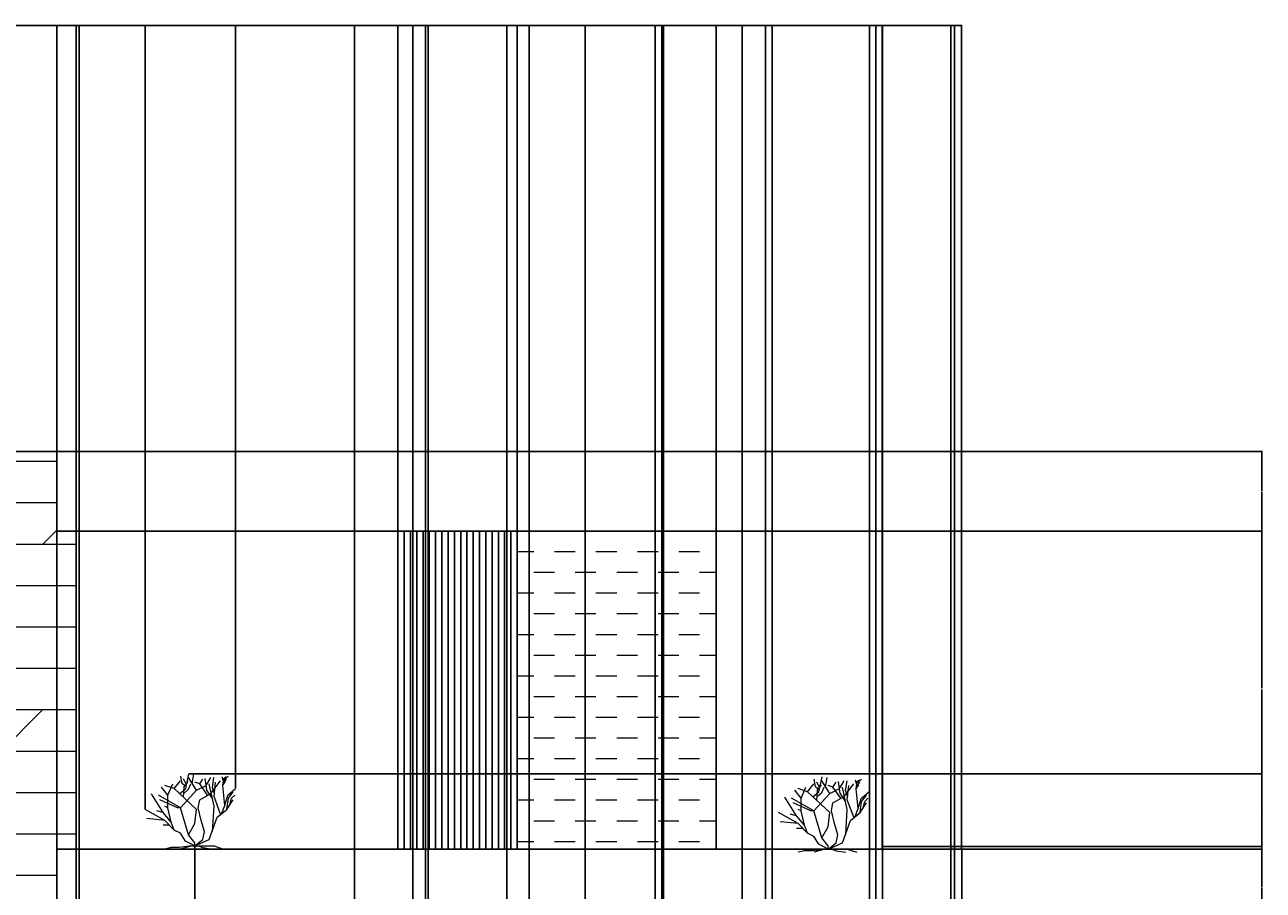
# Model space of a CAD drawing. Units: inches. Extents: x 250 to 1217, y -42 to 832.
# Tile 7 of 7: x 670 to 1043, y 571 to 832. Entities that reach past the tile are written whole.
import ezdxf

# ---------------------------------------------------------------- set-up
doc = ezdxf.new("R2010")
doc.units = ezdxf.units.IN
doc.header["$MEASUREMENT"] = 0
for name, color, linetype, lineweight in [('A-ANNO-DIMS', 2, 'Continuous', 18), ('A-ELEV', 7, 'Continuous', 25), ('A-ELEV-PATT', 8, 'Continuous', 13), ('L-PLNT', 3, 'Continuous', 13)]:
    doc.layers.add(name, color=color, linetype=linetype, lineweight=lineweight)
doc.styles.get("Standard").update_dxf_attribs({"font": 'arial.ttf'})
doc.dimstyles.get("Standard").update_dxf_attribs({"dimtxt": 0.18, "dimasz": 0.18, "dimexe": 0.18, "dimexo": 0.0625, "dimgap": 0.09, "dimtad": 0, "dimtih": 1, "dimtoh": 1, "dimdec": 4, "dimzin": 0, "dimdsep": 46, "dimtxsty": 'Standard', "dimcen": 0.09, "dimadec": 0, "dimazin": 0, "dimtfac": 1, "dimtdec": 4, "dimtofl": 0, "dimtmove": 0, "dimatfit": 3, "dimfxl": 1, "dimtolj": 1, "dimtzin": 0, "dimarcsym": 0})

# ---------------------------------------------------------------- blocks, each defined once
blk = doc.blocks.new('*U2')
for p, q in [((-11.433, 18.289), (-10.457, 22.749)), ((-9.48, 19.775), (-8.992, 22.592)), ((-16.8, 16.32), (-18.72, 18.72)), ((-14.88, 18.24), (-17.76, 19.2)), ((-16.8, 16.32), (-15.36, 19.68)), ((-14.88, 18.24), (-12.96, 20.64)), ((-12.471, 19.775), (-12.898, 22.044)), ((-11.677, 19.071), (-12.471, 19.775)), ((-11.28, 19.619), (-12.104, 21.184)), ((-12.043, 15.628), (-11.921, 18.836)), ((-11.921, 18.836), (-10.64, 20.401)), ((-10.579, 18.054), (-9.846, 19.697)), ((-8.16, 17.76), (-10.56, 21.6)), ((-7.2, 19.68), (-8.64, 20.16)), ((-8.16, 17.76), (-5.28, 19.2)), ((-7.2, 19.68), (-6.24, 21.12)), ((-4.8, 16.32), (-7.2, 19.68)), ((-5.086, 17.741), (-5.513, 21.34)), ((-5.28, 19.2), (-3.84, 21.6)), ((-2.88, 12.96), (-4.32, 19.68)), ((-3.84, 16.8), (-0.96, 20.64)), ((-3.377, 18.602), (-2.888, 21.575)), ((-2.88, 15.84), (-2.4, 20.16)), ((-0.508, 21.888), (-0.081, 20.558)), ((-0.203, 19.149), (0.102, 21.34)), ((0.346, 13.203), (-0.203, 19.149)), ((-0.142, 19.384), (0.59, 20.401)), ((-0.02, 20.01), (0.896, 21.105)), ((0.041, 20.714), (1.384, 22.044)), ((0.102, 21.34), (0.835, 21.888)), ((-18.24, 11.04), (-21.755, 16.655)), ((-12.96, 12.48), (-19.68, 16.32)), ((-16.8, 12.48), (-16.8, 16.32)), ((-8.16, 12), (-14.88, 18.24)), ((-13.325, 16.724), (-11.433, 18.289)), ((-12.96, 12.48), (-8.16, 17.76)), ((-11.982, 16.802), (-10.579, 18.054)), ((-7.2, 14.88), (-3.84, 16.8)), ((-3.377, 15.315), (-5.086, 17.819)), ((-2.766, 16.802), (-3.377, 18.602)), ((-0.96, 10.56), (-2.88, 15.84)), ((0.346, 13.203), (1.323, 16.254)), ((0.96, 12), (1.44, 15.36)), ((1.323, 16.254), (3.642, 18.289)), ((1.44, 15.36), (2.88, 17.28)), ((1.92, 13.44), (2.4, 15.36)), ((2.4, 15.36), (3.36, 16.32)), ((-17.76, 8.64), (-23.663, 11.961)), ((-18.24, 11.04), (-20.16, 11.52)), ((-13.92, 12.48), (-19.2, 14.88)), ((-16.8, 12.48), (-17.76, 12.96)), ((-15.84, 8.16), (-16.8, 12.48)), ((-12.96, 12.48), (-13.92, 12.48)), ((-10.56, 4.32), (-12.96, 12.48)), ((-8.64, 7.68), (-8.16, 12)), ((-7.68, 12.48), (-7.2, 14.88)), ((-6.72, 8.64), (-7.68, 12.48)), ((-3.36, 5.28), (-2.88, 12.96)), ((-1.92, 9.6), (0.96, 12)), ((-0.48, 10.8), (0.346, 13.203)), ((0.96, 12), (2.88, 14.88)), ((-17.76, 8.64), (-23.128, 9.222)), ((-15.84, 8.16), (-18.24, 11.04)), ((-14.88, 5.76), (-17.76, 8.64)), ((-14.88, 5.76), (-15.84, 8.16)), ((-10.56, 4.32), (-8.64, 7.68)), ((-5.76, 5.28), (-6.72, 8.64)), ((-4.32, 2.88), (-1.92, 9.6)), ((-16.32, 7.2), (-18.24, 7.2)), ((-12.96, 4.8), (-14.88, 5.76)), ((-11.52, 2.4), (-12.96, 4.8)), ((-8.64, 1.92), (-10.56, 4.32)), ((-6.24, 2.88), (-5.76, 5.28)), ((-15.84, 0.48), (-17.76, 0)), ((-13.44, 0.48), (-15.84, 0.48)), ((-9.6, 0.96), (-13.44, 0.48)), ((-9.6, 0.96), (-12.96, 0)), ((-8.64, 0.96), (-11.52, 2.4)), ((-9.6, 0.96), (-7.68, 0.96)), ((-8.64, 0.96), (-4.32, 2.88)), ((-8.64, 0.96), (-6.24, 2.88)), ((-8.64, 0.96), (-8.64, 1.92)), ((-8.64, 0.96), (-2.88, 0.96)), ((-7.68, 0.96), (-6.24, 0.48)), ((-6.24, 0.48), (-3.36, 0)), ((-2.88, 0.96), (0, 0))]:
    blk.add_line(p, q)
blk = doc.blocks.new('*D9')
at = {"layer": 'A-ANNO-DIMS', "color": 0, "lineweight": -2, "transparency": 16777216}
for p, q in [((630.78, 702.99), (630.78, 831.77)), ((630.96, 831.59), (654.6, 831.59)), ((679.01, 831.59), (655.36, 831.59)), ((679.19, 702.99), (679.19, 831.77))]:
    blk.add_line(p, q, dxfattribs=at)
at = {"layer": 'A-ANNO-DIMS', "color": 0, "transparency": 16777216}
for points in [[(630.96, 831.62), (630.96, 831.56), (630.78, 831.59)], [(679.01, 831.62), (679.01, 831.56), (679.19, 831.59)]]:
    blk.add_solid(points, dxfattribs=at)
at = {"layer": 'Defpoints', "color": 0, "transparency": 16777216}
for p in [(679.19, 831.59), (630.78, 702.93), (679.19, 702.93)]:
    blk.add_point(p, dxfattribs=at)
at = {"layer": 'A-ANNO-DIMS', "color": 0, "transparency": 16777216, "insert": (654.98, 831.59), "char_height": 0.18, "attachment_point": 5}
blk.add_mtext('\\A1;48.41', dxfattribs=at)
blk = doc.blocks.new('*D10')
at = {"layer": 'A-ANNO-DIMS', "color": 0, "lineweight": -2, "transparency": 16777216}
for p, q in [((679.19, 702.99), (679.19, 831.77)), ((679.37, 831.59), (815.24, 831.59)), ((952.05, 831.59), (816.18, 831.59)), ((952.23, 702.99), (952.23, 831.77))]:
    blk.add_line(p, q, dxfattribs=at)
at = {"layer": 'A-ANNO-DIMS', "color": 0, "transparency": 16777216}
for points in [[(679.37, 831.62), (679.37, 831.56), (679.19, 831.59)], [(952.05, 831.62), (952.05, 831.56), (952.23, 831.59)]]:
    blk.add_solid(points, dxfattribs=at)
at = {"layer": 'Defpoints', "color": 0, "transparency": 16777216}
for p in [(952.23, 831.59), (679.19, 702.93), (952.23, 702.93)]:
    blk.add_point(p, dxfattribs=at)
at = {"layer": 'A-ANNO-DIMS', "color": 0, "transparency": 16777216, "insert": (815.71, 831.59), "char_height": 0.18, "attachment_point": 5}
blk.add_mtext('\\A1;273.05', dxfattribs=at)
blk = doc.blocks.new('*D19')
at = {"layer": 'A-ANNO-DIMS', "color": 0, "lineweight": -2, "transparency": 16777216}
for p, q in [((928.21, 583.67), (1043.08, 583.67)), ((1042.9, 583.49), (1042.9, 571.48)), ((1042.9, 559.11), (1042.9, 571.12)), ((952.41, 558.93), (1043.08, 558.93))]:
    blk.add_line(p, q, dxfattribs=at)
at = {"layer": 'A-ANNO-DIMS', "color": 0, "transparency": 16777216}
for points in [[(1042.87, 583.49), (1042.93, 583.49), (1042.9, 583.67)], [(1042.87, 559.11), (1042.93, 559.11), (1042.9, 558.93)]]:
    blk.add_solid(points, dxfattribs=at)
at = {"layer": 'Defpoints', "color": 0, "transparency": 16777216}
for p in [(928.15, 583.67), (1042.9, 583.67), (952.34, 558.93)]:
    blk.add_point(p, dxfattribs=at)
at = {"layer": 'A-ANNO-DIMS', "color": 0, "transparency": 16777216, "insert": (1042.9, 571.3), "char_height": 0.18, "attachment_point": 5}
blk.add_mtext('\\A1;24.747', dxfattribs=at)
blk = doc.blocks.new('*D20')
at = {"layer": 'A-ANNO-DIMS', "color": 0, "lineweight": -2, "transparency": 16777216}
for p, q in [((928.3, 678.93), (1043.08, 678.93)), ((1042.9, 678.75), (1042.9, 631.48)), ((1042.9, 583.85), (1042.9, 631.12)), ((928.21, 583.67), (1043.08, 583.67))]:
    blk.add_line(p, q, dxfattribs=at)
at = {"layer": 'A-ANNO-DIMS', "color": 0, "transparency": 16777216}
for points in [[(1042.87, 678.75), (1042.93, 678.75), (1042.9, 678.93)], [(1042.87, 583.85), (1042.93, 583.85), (1042.9, 583.67)]]:
    blk.add_solid(points, dxfattribs=at)
at = {"layer": 'Defpoints', "color": 0, "transparency": 16777216}
for p in [(928.23, 678.93), (1042.9, 678.93), (928.15, 583.67)]:
    blk.add_point(p, dxfattribs=at)
at = {"layer": 'A-ANNO-DIMS', "color": 0, "transparency": 16777216, "insert": (1042.9, 631.3), "char_height": 0.18, "attachment_point": 5}
blk.add_mtext('\\A1;95.25', dxfattribs=at)
blk = doc.blocks.new('*D21')
at = {"layer": 'A-ANNO-DIMS', "color": 0, "lineweight": -2, "transparency": 16777216}
for p, q in [((952.3, 702.93), (1043.08, 702.93)), ((1042.9, 702.75), (1042.9, 691.11)), ((1042.9, 679.11), (1042.9, 690.75)), ((928.3, 678.93), (1043.08, 678.93))]:
    blk.add_line(p, q, dxfattribs=at)
at = {"layer": 'A-ANNO-DIMS', "color": 0, "transparency": 16777216}
for points in [[(1042.87, 702.75), (1042.93, 702.75), (1042.9, 702.93)], [(1042.87, 679.11), (1042.93, 679.11), (1042.9, 678.93)]]:
    blk.add_solid(points, dxfattribs=at)
at = {"layer": 'Defpoints', "color": 0, "transparency": 16777216}
for p in [(952.23, 702.93), (1042.9, 702.93), (928.23, 678.93)]:
    blk.add_point(p, dxfattribs=at)
at = {"layer": 'A-ANNO-DIMS', "color": 0, "transparency": 16777216, "insert": (1042.9, 690.93), "char_height": 0.18, "attachment_point": 5}
blk.add_mtext('\\A1;24', dxfattribs=at)
blk = doc.blocks.new('*D27')
at = {"layer": 'A-ANNO-DIMS', "color": 0, "lineweight": -2, "transparency": 16777216}
for p, q in [((624.98, 174.99), (624.98, 831.77)), ((625.16, 831.59), (655.07, 831.59)), ((685.76, 831.59), (655.86, 831.59)), ((685.94, 176.49), (685.94, 831.77))]:
    blk.add_line(p, q, dxfattribs=at)
at = {"layer": 'A-ANNO-DIMS', "color": 0, "transparency": 16777216}
for points in [[(625.16, 831.62), (625.16, 831.56), (624.98, 831.59)], [(685.76, 831.62), (685.76, 831.56), (685.94, 831.59)]]:
    blk.add_solid(points, dxfattribs=at)
at = {"layer": 'Defpoints', "color": 0, "transparency": 16777216}
for p in [(685.94, 831.59), (685.94, 176.43), (624.98, 174.93)]:
    blk.add_point(p, dxfattribs=at)
at = {"layer": 'A-ANNO-DIMS', "color": 0, "transparency": 16777216, "insert": (655.46, 831.59), "char_height": 0.18, "attachment_point": 5}
blk.add_mtext('\\A1;60.96', dxfattribs=at)
blk = doc.blocks.new('*D28')
at = {"layer": 'A-ANNO-DIMS', "color": 0, "lineweight": -2, "transparency": 16777216}
for p, q in [((685.94, 176.49), (685.94, 831.77)), ((686.12, 831.59), (727.07, 831.59)), ((768.8, 831.59), (727.86, 831.59)), ((768.98, 162.99), (768.98, 831.77))]:
    blk.add_line(p, q, dxfattribs=at)
at = {"layer": 'A-ANNO-DIMS', "color": 0, "transparency": 16777216}
for points in [[(686.12, 831.62), (686.12, 831.56), (685.94, 831.59)], [(768.8, 831.62), (768.8, 831.56), (768.98, 831.59)]]:
    blk.add_solid(points, dxfattribs=at)
at = {"layer": 'Defpoints', "color": 0, "transparency": 16777216}
for p in [(768.98, 831.59), (685.94, 176.43), (768.98, 162.93)]:
    blk.add_point(p, dxfattribs=at)
at = {"layer": 'A-ANNO-DIMS', "color": 0, "transparency": 16777216, "insert": (727.46, 831.59), "char_height": 0.18, "attachment_point": 5}
blk.add_mtext('\\A1;83.04', dxfattribs=at)
blk = doc.blocks.new('*D29')
at = {"layer": 'A-ANNO-DIMS', "color": 0, "lineweight": -2, "transparency": 16777216}
for p, q in [((768.98, 162.99), (768.98, 831.77)), ((769.16, 831.59), (779.67, 831.59)), ((791.11, 831.59), (780.6, 831.59)), ((791.29, 174.99), (791.29, 831.77))]:
    blk.add_line(p, q, dxfattribs=at)
at = {"layer": 'A-ANNO-DIMS', "color": 0, "transparency": 16777216}
for points in [[(769.16, 831.62), (769.16, 831.56), (768.98, 831.59)], [(791.11, 831.62), (791.11, 831.56), (791.29, 831.59)]]:
    blk.add_solid(points, dxfattribs=at)
at = {"layer": 'Defpoints', "color": 0, "transparency": 16777216}
for p in [(791.29, 831.59), (791.29, 174.93), (768.98, 162.93)]:
    blk.add_point(p, dxfattribs=at)
at = {"layer": 'A-ANNO-DIMS', "color": 0, "transparency": 16777216, "insert": (780.13, 831.59), "char_height": 0.18, "attachment_point": 5}
blk.add_mtext('\\A1;22.303', dxfattribs=at)
blk = doc.blocks.new('*D30')
at = {"layer": 'A-ANNO-DIMS', "color": 0, "lineweight": -2, "transparency": 16777216}
for p, q in [((814.96, 174.99), (814.96, 831.77)), ((815.14, 831.59), (826.33, 831.59)), ((838.45, 831.59), (827.26, 831.59)), ((838.63, 174.99), (838.63, 831.77))]:
    blk.add_line(p, q, dxfattribs=at)
at = {"layer": 'A-ANNO-DIMS', "color": 0, "transparency": 16777216}
for points in [[(815.14, 831.62), (815.14, 831.56), (814.96, 831.59)], [(838.45, 831.62), (838.45, 831.56), (838.63, 831.59)]]:
    blk.add_solid(points, dxfattribs=at)
at = {"layer": 'Defpoints', "color": 0, "transparency": 16777216}
for p in [(838.63, 831.59), (814.96, 174.93), (838.63, 174.93)]:
    blk.add_point(p, dxfattribs=at)
at = {"layer": 'A-ANNO-DIMS', "color": 0, "transparency": 16777216, "insert": (826.8, 831.59), "char_height": 0.18, "attachment_point": 5}
blk.add_mtext('\\A1;23.674', dxfattribs=at)
blk = doc.blocks.new('*D31')
at = {"layer": 'A-ANNO-DIMS', "color": 0, "lineweight": -2, "transparency": 16777216}
for p, q in [((862.31, 174.99), (862.31, 831.77)), ((862.49, 831.59), (873.68, 831.59)), ((885.8, 831.59), (874.61, 831.59)), ((885.98, 174.99), (885.98, 831.77))]:
    blk.add_line(p, q, dxfattribs=at)
at = {"layer": 'A-ANNO-DIMS', "color": 0, "transparency": 16777216}
for points in [[(862.49, 831.62), (862.49, 831.56), (862.31, 831.59)], [(885.8, 831.62), (885.8, 831.56), (885.98, 831.59)]]:
    blk.add_solid(points, dxfattribs=at)
at = {"layer": 'Defpoints', "color": 0, "transparency": 16777216}
for p in [(885.98, 831.59), (862.31, 174.93), (885.98, 174.93)]:
    blk.add_point(p, dxfattribs=at)
at = {"layer": 'A-ANNO-DIMS', "color": 0, "transparency": 16777216, "insert": (874.15, 831.59), "char_height": 0.18, "attachment_point": 5}
blk.add_mtext('\\A1;23.674', dxfattribs=at)
blk = doc.blocks.new('*D32')
at = {"layer": 'A-ANNO-DIMS', "color": 0, "lineweight": -2, "transparency": 16777216}
for p, q in [((885.98, 174.99), (885.98, 831.77)), ((886.16, 831.59), (917.26, 831.59)), ((948.8, 831.59), (917.7, 831.59)), ((948.98, 174.99), (948.98, 831.77))]:
    blk.add_line(p, q, dxfattribs=at)
at = {"layer": 'A-ANNO-DIMS', "color": 0, "transparency": 16777216}
for points in [[(886.16, 831.62), (886.16, 831.56), (885.98, 831.59)], [(948.8, 831.62), (948.8, 831.56), (948.98, 831.59)]]:
    blk.add_solid(points, dxfattribs=at)
at = {"layer": 'Defpoints', "color": 0, "transparency": 16777216}
for p in [(948.98, 831.59), (885.98, 174.93), (948.98, 174.93)]:
    blk.add_point(p, dxfattribs=at)
at = {"layer": 'A-ANNO-DIMS', "color": 0, "transparency": 16777216, "insert": (917.48, 831.59), "char_height": 0.18, "attachment_point": 5}
blk.add_mtext('\\A1;63', dxfattribs=at)
blk = doc.blocks.new('*D33')
at = {"layer": 'A-ANNO-DIMS', "color": 0, "lineweight": -2, "transparency": 16777216}
for p, q in [((791.29, 414.99), (791.29, 831.77)), ((791.47, 831.59), (802.66, 831.59)), ((814.78, 831.59), (803.59, 831.59)), ((814.96, 414.99), (814.96, 831.77))]:
    blk.add_line(p, q, dxfattribs=at)
at = {"layer": 'A-ANNO-DIMS', "color": 0, "transparency": 16777216}
for points in [[(791.47, 831.62), (791.47, 831.56), (791.29, 831.59)], [(814.78, 831.62), (814.78, 831.56), (814.96, 831.59)]]:
    blk.add_solid(points, dxfattribs=at)
at = {"layer": 'Defpoints', "color": 0, "transparency": 16777216}
for p in [(814.96, 831.59), (791.29, 414.93), (814.96, 414.93)]:
    blk.add_point(p, dxfattribs=at)
at = {"layer": 'A-ANNO-DIMS', "color": 0, "transparency": 16777216, "insert": (803.12, 831.59), "char_height": 0.18, "attachment_point": 5}
blk.add_mtext('\\A1;23.674', dxfattribs=at)
blk = doc.blocks.new('*D34')
at = {"layer": 'A-ANNO-DIMS', "color": 0, "lineweight": -2, "transparency": 16777216}
for p, q in [((838.63, 414.99), (838.63, 831.77)), ((838.81, 831.59), (850.01, 831.59)), ((862.13, 831.59), (850.94, 831.59)), ((862.31, 414.99), (862.31, 831.77))]:
    blk.add_line(p, q, dxfattribs=at)
at = {"layer": 'A-ANNO-DIMS', "color": 0, "transparency": 16777216}
for points in [[(838.81, 831.62), (838.81, 831.56), (838.63, 831.59)], [(862.13, 831.62), (862.13, 831.56), (862.31, 831.59)]]:
    blk.add_solid(points, dxfattribs=at)
at = {"layer": 'Defpoints', "color": 0, "transparency": 16777216}
for p in [(862.31, 831.59), (838.63, 414.93), (862.31, 414.93)]:
    blk.add_point(p, dxfattribs=at)
at = {"layer": 'A-ANNO-DIMS', "color": 0, "transparency": 16777216, "insert": (850.47, 831.59), "char_height": 0.18, "attachment_point": 5}
blk.add_mtext('\\A1;23.674', dxfattribs=at)
blk = doc.blocks.new('*D45')
at = {"layer": 'A-ANNO-DIMS', "color": 0, "lineweight": -2, "transparency": 16777216}
for p, q in [((685.06, 678.99), (685.06, 831.77)), ((685.24, 831.59), (733.21, 831.59)), ((781.95, 831.59), (733.99, 831.59)), ((782.13, 678.99), (782.13, 831.77))]:
    blk.add_line(p, q, dxfattribs=at)
at = {"layer": 'A-ANNO-DIMS', "color": 0, "transparency": 16777216}
for points in [[(685.24, 831.62), (685.24, 831.56), (685.06, 831.59)], [(781.95, 831.62), (781.95, 831.56), (782.13, 831.59)]]:
    blk.add_solid(points, dxfattribs=at)
at = {"layer": 'Defpoints', "color": 0, "transparency": 16777216}
for p in [(782.13, 831.59), (685.06, 678.93), (782.13, 678.93)]:
    blk.add_point(p, dxfattribs=at)
at = {"layer": 'A-ANNO-DIMS', "color": 0, "transparency": 16777216, "insert": (733.6, 831.59), "char_height": 0.18, "attachment_point": 5}
blk.add_mtext('\\A1;97.07', dxfattribs=at)
blk = doc.blocks.new('*D46')
at = {"layer": 'A-ANNO-DIMS', "color": 0, "lineweight": -2, "transparency": 16777216}
for p, q in [((782.13, 678.99), (782.13, 831.77)), ((782.31, 831.59), (799.91, 831.59)), ((817.95, 831.59), (800.35, 831.59)), ((818.13, 678.99), (818.13, 831.77))]:
    blk.add_line(p, q, dxfattribs=at)
at = {"layer": 'A-ANNO-DIMS', "color": 0, "transparency": 16777216}
for points in [[(782.31, 831.62), (782.31, 831.56), (782.13, 831.59)], [(817.95, 831.62), (817.95, 831.56), (818.13, 831.59)]]:
    blk.add_solid(points, dxfattribs=at)
at = {"layer": 'Defpoints', "color": 0, "transparency": 16777216}
for p in [(818.13, 831.59), (782.13, 678.93), (818.13, 678.93)]:
    blk.add_point(p, dxfattribs=at)
at = {"layer": 'A-ANNO-DIMS', "color": 0, "transparency": 16777216, "insert": (800.13, 831.59), "char_height": 0.18, "attachment_point": 5}
blk.add_mtext('\\A1;36', dxfattribs=at)
blk = doc.blocks.new('*D47')
at = {"layer": 'A-ANNO-DIMS', "color": 0, "lineweight": -2, "transparency": 16777216}
for p, q in [((818.13, 678.99), (818.13, 831.77)), ((818.31, 831.59), (847.91, 831.59)), ((877.95, 831.59), (848.35, 831.59)), ((878.13, 678.99), (878.13, 831.77))]:
    blk.add_line(p, q, dxfattribs=at)
at = {"layer": 'A-ANNO-DIMS', "color": 0, "transparency": 16777216}
for points in [[(818.31, 831.62), (818.31, 831.56), (818.13, 831.59)], [(877.95, 831.62), (877.95, 831.56), (878.13, 831.59)]]:
    blk.add_solid(points, dxfattribs=at)
at = {"layer": 'Defpoints', "color": 0, "transparency": 16777216}
for p in [(878.13, 831.59), (818.13, 678.93), (878.13, 678.93)]:
    blk.add_point(p, dxfattribs=at)
at = {"layer": 'A-ANNO-DIMS', "color": 0, "transparency": 16777216, "insert": (848.13, 831.59), "char_height": 0.18, "attachment_point": 5}
blk.add_mtext('\\A1;60', dxfattribs=at)
blk = doc.blocks.new('*D48')
at = {"layer": 'A-ANNO-DIMS', "color": 0, "lineweight": -2, "transparency": 16777216}
for p, q in [((878.13, 678.99), (878.13, 831.77)), ((878.31, 831.59), (902.88, 831.59)), ((928.05, 831.59), (903.49, 831.59)), ((928.23, 678.99), (928.23, 831.77))]:
    blk.add_line(p, q, dxfattribs=at)
at = {"layer": 'A-ANNO-DIMS', "color": 0, "transparency": 16777216}
for points in [[(878.31, 831.62), (878.31, 831.56), (878.13, 831.59)], [(928.05, 831.62), (928.05, 831.56), (928.23, 831.59)]]:
    blk.add_solid(points, dxfattribs=at)
at = {"layer": 'Defpoints', "color": 0, "transparency": 16777216}
for p in [(928.23, 831.59), (878.13, 678.93), (928.23, 678.93)]:
    blk.add_point(p, dxfattribs=at)
at = {"layer": 'A-ANNO-DIMS', "color": 0, "transparency": 16777216, "insert": (903.18, 831.59), "char_height": 0.18, "attachment_point": 5}
blk.add_mtext('\\A1;50.1', dxfattribs=at)
blk = doc.blocks.new('*D50')
at = {"layer": 'A-ANNO-DIMS', "color": 0, "lineweight": -2, "transparency": 16777216}
for p, q in [((679.19, 318.99), (679.19, 831.77)), ((679.37, 831.59), (814.16, 831.59)), ((949.88, 831.59), (815.09, 831.59)), ((950.06, 318.99), (950.06, 831.77))]:
    blk.add_line(p, q, dxfattribs=at)
at = {"layer": 'A-ANNO-DIMS', "color": 0, "transparency": 16777216}
for points in [[(679.37, 831.62), (679.37, 831.56), (679.19, 831.59)], [(949.88, 831.62), (949.88, 831.56), (950.06, 831.59)]]:
    blk.add_solid(points, dxfattribs=at)
at = {"layer": 'Defpoints', "color": 0, "transparency": 16777216}
for p in [(950.06, 831.59), (679.19, 318.93), (950.06, 318.93)]:
    blk.add_point(p, dxfattribs=at)
at = {"layer": 'A-ANNO-DIMS', "color": 0, "transparency": 16777216, "insert": (814.62, 831.59), "char_height": 0.18, "attachment_point": 5}
blk.add_mtext('\\A1;270.87', dxfattribs=at)
blk = doc.blocks.new('*D52')
at = {"layer": 'A-ANNO-DIMS', "color": 0, "lineweight": -2, "transparency": 16777216}
for p, q in [((924.49, 199.65), (924.49, 831.77)), ((924.67, 831.59), (936.34, 831.59)), ((948.8, 831.59), (937.13, 831.59)), ((948.98, 198.99), (948.98, 831.77))]:
    blk.add_line(p, q, dxfattribs=at)
at = {"layer": 'A-ANNO-DIMS', "color": 0, "transparency": 16777216}
for points in [[(924.67, 831.62), (924.67, 831.56), (924.49, 831.59)], [(948.8, 831.62), (948.8, 831.56), (948.98, 831.59)]]:
    blk.add_solid(points, dxfattribs=at)
at = {"layer": 'Defpoints', "color": 0, "transparency": 16777216}
for p in [(948.98, 831.59), (924.49, 199.59), (948.98, 198.93)]:
    blk.add_point(p, dxfattribs=at)
at = {"layer": 'A-ANNO-DIMS', "color": 0, "transparency": 16777216, "insert": (936.74, 831.59), "char_height": 0.18, "attachment_point": 5}
blk.add_mtext('\\A1;24.49', dxfattribs=at)
blk = doc.blocks.new('*D55')
at = {"layer": 'A-ANNO-DIMS', "color": 0, "lineweight": -2, "transparency": 16777216}
for p, q in [((684.98, 438.99), (684.98, 831.77)), ((685.16, 831.59), (735.35, 831.59)), ((786.44, 831.59), (736.26, 831.59)), ((786.62, 438.99), (786.62, 831.77))]:
    blk.add_line(p, q, dxfattribs=at)
at = {"layer": 'A-ANNO-DIMS', "color": 0, "transparency": 16777216}
for points in [[(685.16, 831.62), (685.16, 831.56), (684.98, 831.59)], [(786.44, 831.62), (786.44, 831.56), (786.62, 831.59)]]:
    blk.add_solid(points, dxfattribs=at)
at = {"layer": 'Defpoints', "color": 0, "transparency": 16777216}
for p in [(786.62, 831.59), (684.98, 438.93), (786.62, 438.93)]:
    blk.add_point(p, dxfattribs=at)
at = {"layer": 'A-ANNO-DIMS', "color": 0, "transparency": 16777216, "insert": (735.8, 831.59), "char_height": 0.18, "attachment_point": 5}
blk.add_mtext('\\A1;101.64', dxfattribs=at)
blk = doc.blocks.new('*D56')
at = {"layer": 'A-ANNO-DIMS', "color": 0, "lineweight": -2, "transparency": 16777216}
for p, q in [((786.62, 438.99), (786.62, 831.77)), ((786.8, 831.59), (803.8, 831.59)), ((821.58, 831.59), (804.59, 831.59)), ((821.76, 438.99), (821.76, 831.77))]:
    blk.add_line(p, q, dxfattribs=at)
at = {"layer": 'A-ANNO-DIMS', "color": 0, "transparency": 16777216}
for points in [[(786.8, 831.62), (786.8, 831.56), (786.62, 831.59)], [(821.58, 831.62), (821.58, 831.56), (821.76, 831.59)]]:
    blk.add_solid(points, dxfattribs=at)
at = {"layer": 'Defpoints', "color": 0, "transparency": 16777216}
for p in [(821.76, 831.59), (786.62, 438.93), (821.76, 438.93)]:
    blk.add_point(p, dxfattribs=at)
at = {"layer": 'A-ANNO-DIMS', "color": 0, "transparency": 16777216, "insert": (804.19, 831.59), "char_height": 0.18, "attachment_point": 5}
blk.add_mtext('\\A1;35.14', dxfattribs=at)
blk = doc.blocks.new('*D57')
at = {"layer": 'A-ANNO-DIMS', "color": 0, "lineweight": -2, "transparency": 16777216}
for p, q in [((821.76, 438.99), (821.76, 831.77)), ((821.94, 831.59), (840.54, 831.59)), ((859.58, 831.59), (840.98, 831.59)), ((859.76, 438.99), (859.76, 831.77))]:
    blk.add_line(p, q, dxfattribs=at)
at = {"layer": 'A-ANNO-DIMS', "color": 0, "transparency": 16777216}
for points in [[(821.94, 831.62), (821.94, 831.56), (821.76, 831.59)], [(859.58, 831.62), (859.58, 831.56), (859.76, 831.59)]]:
    blk.add_solid(points, dxfattribs=at)
at = {"layer": 'Defpoints', "color": 0, "transparency": 16777216}
for p in [(859.76, 831.59), (821.76, 438.93), (859.76, 438.93)]:
    blk.add_point(p, dxfattribs=at)
at = {"layer": 'A-ANNO-DIMS', "color": 0, "transparency": 16777216, "insert": (840.76, 831.59), "char_height": 0.18, "attachment_point": 5}
blk.add_mtext('\\A1;38', dxfattribs=at)
blk = doc.blocks.new('*D58')
at = {"layer": 'A-ANNO-DIMS', "color": 0, "lineweight": -2, "transparency": 16777216}
for p, q in [((859.76, 438.99), (859.76, 831.77)), ((859.94, 831.59), (893.74, 831.59)), ((928.18, 831.59), (894.39, 831.59)), ((928.36, 438.99), (928.36, 831.77))]:
    blk.add_line(p, q, dxfattribs=at)
at = {"layer": 'A-ANNO-DIMS', "color": 0, "transparency": 16777216}
for points in [[(859.94, 831.62), (859.94, 831.56), (859.76, 831.59)], [(928.18, 831.62), (928.18, 831.56), (928.36, 831.59)]]:
    blk.add_solid(points, dxfattribs=at)
at = {"layer": 'Defpoints', "color": 0, "transparency": 16777216}
for p in [(928.36, 831.59), (859.76, 438.93), (928.36, 438.93)]:
    blk.add_point(p, dxfattribs=at)
at = {"layer": 'A-ANNO-DIMS', "color": 0, "transparency": 16777216, "insert": (894.06, 831.59), "char_height": 0.18, "attachment_point": 5}
blk.add_mtext('\\A1;68.6', dxfattribs=at)
blk = doc.blocks.new('*D87')
at = {"layer": 'A-ANNO-DIMS', "color": 0, "lineweight": -2, "transparency": 16777216}
for p, q in [((790.46, 438.99), (790.46, 831.77)), ((790.64, 831.59), (805.72, 831.59)), ((821.58, 831.59), (806.51, 831.59)), ((821.76, 438.99), (821.76, 831.77))]:
    blk.add_line(p, q, dxfattribs=at)
at = {"layer": 'A-ANNO-DIMS', "color": 0, "transparency": 16777216}
for points in [[(790.64, 831.62), (790.64, 831.56), (790.46, 831.59)], [(821.58, 831.62), (821.58, 831.56), (821.76, 831.59)]]:
    blk.add_solid(points, dxfattribs=at)
at = {"layer": 'Defpoints', "color": 0, "transparency": 16777216}
for p in [(821.76, 831.59), (790.46, 438.93), (821.76, 438.93)]:
    blk.add_point(p, dxfattribs=at)
at = {"layer": 'A-ANNO-DIMS', "color": 0, "transparency": 16777216, "insert": (806.11, 831.59), "char_height": 0.18, "attachment_point": 5}
blk.add_mtext('\\A1;31.30', dxfattribs=at)
blk = doc.blocks.new('*D88')
at = {"layer": 'A-ANNO-DIMS', "color": 0, "lineweight": -2, "transparency": 16777216}
for p, q in [((861.76, 438.99), (861.76, 831.77)), ((861.94, 831.59), (877.02, 831.59)), ((892.88, 831.59), (877.81, 831.59)), ((893.06, 438.99), (893.06, 831.77))]:
    blk.add_line(p, q, dxfattribs=at)
at = {"layer": 'A-ANNO-DIMS', "color": 0, "transparency": 16777216}
for points in [[(861.94, 831.62), (861.94, 831.56), (861.76, 831.59)], [(892.88, 831.62), (892.88, 831.56), (893.06, 831.59)]]:
    blk.add_solid(points, dxfattribs=at)
at = {"layer": 'Defpoints', "color": 0, "transparency": 16777216}
for p in [(893.06, 831.59), (861.76, 438.93), (893.06, 438.93)]:
    blk.add_point(p, dxfattribs=at)
at = {"layer": 'A-ANNO-DIMS', "color": 0, "transparency": 16777216, "insert": (877.41, 831.59), "char_height": 0.18, "attachment_point": 5}
blk.add_mtext('\\A1;31.30', dxfattribs=at)
blk = doc.blocks.new('*D89')
at = {"layer": 'A-ANNO-DIMS', "color": 0, "lineweight": -2, "transparency": 16777216}
for p, q in [((893.06, 438.99), (893.06, 831.77)), ((893.24, 831.59), (893.74, 831.59)), ((894.88, 831.59), (894.39, 831.59)), ((895.06, 438.99), (895.06, 831.77))]:
    blk.add_line(p, q, dxfattribs=at)
at = {"layer": 'A-ANNO-DIMS', "color": 0, "transparency": 16777216}
for points in [[(893.24, 831.62), (893.24, 831.56), (893.06, 831.59)], [(894.88, 831.62), (894.88, 831.56), (895.06, 831.59)]]:
    blk.add_solid(points, dxfattribs=at)
at = {"layer": 'Defpoints', "color": 0, "transparency": 16777216}
for p in [(895.06, 831.59), (893.06, 438.93), (895.06, 438.93)]:
    blk.add_point(p, dxfattribs=at)
at = {"layer": 'A-ANNO-DIMS', "color": 0, "transparency": 16777216, "insert": (894.06, 831.59), "char_height": 0.18, "attachment_point": 5}
blk.add_mtext('\\A1;2.00', dxfattribs=at)
blk = doc.blocks.new('*D90')
at = {"layer": 'A-ANNO-DIMS', "color": 0, "lineweight": -2, "transparency": 16777216}
for p, q in [((895.06, 438.99), (895.06, 831.77)), ((895.24, 831.59), (910.32, 831.59)), ((926.18, 831.59), (911.11, 831.59)), ((926.36, 438.99), (926.36, 831.77))]:
    blk.add_line(p, q, dxfattribs=at)
at = {"layer": 'A-ANNO-DIMS', "color": 0, "transparency": 16777216}
for points in [[(895.24, 831.62), (895.24, 831.56), (895.06, 831.59)], [(926.18, 831.62), (926.18, 831.56), (926.36, 831.59)]]:
    blk.add_solid(points, dxfattribs=at)
at = {"layer": 'Defpoints', "color": 0, "transparency": 16777216}
for p in [(926.36, 831.59), (895.06, 438.93), (926.36, 438.93)]:
    blk.add_point(p, dxfattribs=at)
at = {"layer": 'A-ANNO-DIMS', "color": 0, "transparency": 16777216, "insert": (910.71, 831.59), "char_height": 0.18, "attachment_point": 5}
blk.add_mtext('\\A1;31.30', dxfattribs=at)
blk = doc.blocks.new('*D96')
at = {"layer": 'A-ANNO-DIMS', "color": 0, "lineweight": -2, "transparency": 16777216}
for p, q in [((705.85, 594.95), (705.85, 831.77)), ((706.03, 831.59), (719.04, 831.59)), ((732.97, 831.59), (719.97, 831.59)), ((733.15, 601.28), (733.15, 831.77))]:
    blk.add_line(p, q, dxfattribs=at)
at = {"layer": 'A-ANNO-DIMS', "color": 0, "transparency": 16777216}
for points in [[(706.03, 831.62), (706.03, 831.56), (705.85, 831.59)], [(732.97, 831.62), (732.97, 831.56), (733.15, 831.59)]]:
    blk.add_solid(points, dxfattribs=at)
at = {"layer": 'Defpoints', "color": 0, "transparency": 16777216}
for p in [(733.15, 831.59), (733.15, 601.22), (705.85, 594.89)]:
    blk.add_point(p, dxfattribs=at)
at = {"layer": 'A-ANNO-DIMS', "color": 0, "transparency": 16777216, "insert": (719.5, 831.59), "char_height": 0.18, "attachment_point": 5}
blk.add_mtext('\\A1;27.305', dxfattribs=at)
blk = doc.blocks.new('*D97')
at = {"layer": 'A-ANNO-DIMS', "color": 0, "lineweight": -2, "transparency": 16777216}
for p, q in [((719.12, 605.68), (1043.08, 605.68)), ((1042.9, 605.5), (1042.9, 594.48)), ((1042.9, 583.11), (1042.9, 594.12)), ((729.57, 582.93), (1043.08, 582.93))]:
    blk.add_line(p, q, dxfattribs=at)
at = {"layer": 'A-ANNO-DIMS', "color": 0, "transparency": 16777216}
for points in [[(1042.87, 605.5), (1042.93, 605.5), (1042.9, 605.68)], [(1042.87, 583.11), (1042.93, 583.11), (1042.9, 582.93)]]:
    blk.add_solid(points, dxfattribs=at)
at = {"layer": 'Defpoints', "color": 0, "transparency": 16777216}
for p in [(719.06, 605.68), (1042.9, 605.68), (729.51, 582.93)]:
    blk.add_point(p, dxfattribs=at)
at = {"layer": 'A-ANNO-DIMS', "color": 0, "transparency": 16777216, "insert": (1042.9, 594.3), "char_height": 0.18, "attachment_point": 5}
blk.add_mtext('\\A1;22.75', dxfattribs=at)
blk = doc.blocks.new('*D98')
at = {"layer": 'A-ANNO-DIMS', "color": 0, "lineweight": -2, "transparency": 16777216}
for p, q in [((720.87, 583.82), (720.87, -41.6)), ((685.06, 582.86), (685.06, -41.6)), ((685.24, -41.42), (702.59, -41.42)), ((720.69, -41.42), (703.34, -41.42))]:
    blk.add_line(p, q, dxfattribs=at)
at = {"layer": 'A-ANNO-DIMS', "color": 0, "transparency": 16777216}
for points in [[(685.24, -41.39), (685.24, -41.45), (685.06, -41.42)], [(720.69, -41.39), (720.69, -41.45), (720.87, -41.42)]]:
    blk.add_solid(points, dxfattribs=at)
at = {"layer": 'Defpoints', "color": 0, "transparency": 16777216}
for p in [(720.87, 583.89), (685.06, 582.93), (720.87, -41.42)]:
    blk.add_point(p, dxfattribs=at)
at = {"layer": 'A-ANNO-DIMS', "color": 0, "transparency": 16777216, "insert": (702.97, -41.42), "char_height": 0.18, "attachment_point": 5}
blk.add_mtext('\\A1;35.81', dxfattribs=at)

msp = doc.modelspace()

# ---------------------------------------------------------------- hatches: boundary and pattern name
at = {"layer": 'A-ELEV-PATT'}
h = msp.add_hatch(dxfattribs=at)
h.set_pattern_fill('DOLMIT', color=256, scale=50)
h.paths.add_polyline_path([(684.9826, 558.9271), (679.1872, 558.9271), (679.1872, 582.9271), (685.0649, 582.9271), (685.0649, 678.9271), (679.1872, 678.9271), (679.1872, 702.9271), (630.7779, 702.9271), (630.7779, 678.9271), (625.0649, 678.9271), (625.0649, 582.9271), (630.7779, 582.9271), (630.7779, 558.9271), (624.9826, 558.9271), (624.9826, 438.9271), (630.7779, 438.9271), (630.7779, 414.9271), (624.9826, 414.9271), (624.9826, 318.9271), (630.7779, 318.9271), (630.7779, 294.9271), (624.9826, 294.9271), (624.9826, 198.9271), (630.7779, 198.9271), (630.7779, 174.9271), (624.9826, 174.9271), (624.9826, 78.9271), (684.9826, 78.9271), (684.9826, 174.9271), (679.1872, 174.9271), (679.1872, 198.9271), (683.6004, 198.9271), (684.9826, 198.9271), (684.9826, 294.9271), (679.1872, 294.9271), (679.1872, 318.9271), (684.9826, 318.9271), (684.9826, 414.9271), (679.1872, 414.9271), (679.1872, 438.9271), (684.9826, 438.9271)])
h = msp.add_hatch(dxfattribs=at)
h.set_pattern_fill('DASH', color=256, scale=50)
h.set_pattern_definition([(0, (373.1506, 504), (6.25, 6.25), [6.25, -6.25])])
h.paths.add_polyline_path([(878.1332, 678.9271), (818.1332, 678.9271), (818.1332, 582.9271), (878.1332, 582.9271)])

# ---------------------------------------------------------------- linework, layer by layer
at = {"layer": 'A-ELEV'}
for p, q in [((679.1872, 702.9271), (679.1872, 678.9271)), ((685.0649, 678.9271), (685.0649, 582.9271)), ((782.1332, 678.9271), (782.1332, 582.9271)), ((784.0279, 678.9271), (784.0279, 582.9271)), ((785.9227, 678.9271), (785.9227, 582.9271)), ((787.8174, 678.9271), (787.8174, 582.9271)), ((789.7121, 678.9271), (789.7121, 582.9271)), ((791.6069, 678.9271), (791.6069, 582.9271)), ((793.5016, 678.9271), (793.5016, 582.9271)), ((795.3963, 678.9271), (795.3963, 582.9271)), ((797.2911, 678.9271), (797.2911, 582.9271)), ((799.1858, 678.9271), (799.1858, 582.9271)), ((801.0806, 678.9271), (801.0806, 582.9271)), ((802.9753, 678.9271), (802.9753, 582.9271)), ((804.87, 678.9271), (804.87, 582.9271)), ((806.7648, 678.9271), (806.7648, 582.9271)), ((808.6595, 678.9271), (808.6595, 582.9271)), ((810.5542, 678.9271), (810.5542, 582.9271)), ((812.449, 678.9271), (812.449, 582.9271)), ((814.3437, 678.9271), (814.3437, 582.9271)), ((816.2384, 678.9271), (816.2384, 582.9271)), ((818.1332, 678.9271), (818.1332, 582.9271)), ((818.1332, 678.9271), (818.1332, 582.9271)), ((818.1332, 678.9271), (818.1332, 582.9271)), ((818.1332, 678.9271), (818.1332, 582.9271)), ((878.1332, 678.9271), (878.1332, 582.9271)), ((679.1872, 582.9271), (679.1872, 558.9271)), ((679.1872, 582.9271), (928.2329, 582.9271)), ((679.1872, 582.9271), (928.2329, 582.9271)), ((952.2329, 582.9271), (952.3429, 582.9271)), ((952.3429, 558.9271), (952.3429, 582.9271))]:
    msp.add_line(p, q, dxfattribs=at)
for points in [[(952.2329, 582.9271), (952.2329, 702.9271), (352.3429, 702.9271), (352.3429, 582.9271)], [(928.2329, 582.9271), (928.2329, 678.9271), (679.1872, 678.9271)]]:
    msp.add_lwpolyline(points, dxfattribs=at)

# ---------------------------------------------------------------- block references
at = {"layer": 'L-PLNT'}
for p in [(729.5123, 582.9271), (920.6336, 581.9671)]:
    msp.add_blockref('*U2', p, dxfattribs=at)

# ---------------------------------------------------------------- dimensions: what is measured, and where the dimension line sits
at = {"layer": 'A-ANNO-DIMS'}
for base, p1, p2, override, picture, middle in [((685.944, 831.5941), (624.9826, 174.9271), (685.944, 176.4321), {"dimdec": 2, "dimlfac": 1, "dimrnd": 0, "dimzin": 0, "dimdsep": 46, "dimlunit": 2}, '*D27', (655.4633, 831.5941)), ((679.1872, 831.5941), (630.7779, 702.9271), (679.1872, 702.9271), {"dimdec": 2, "dimlfac": 1, "dimrnd": 0, "dimzin": 0, "dimdsep": 46, "dimlunit": 2}, '*D9', (654.9826, 831.5941)), ((952.2329, 831.5941), (679.1872, 702.9271), (952.2329, 702.9271), {"dimdec": 2, "dimlfac": 1, "dimrnd": 0, "dimzin": 0, "dimdsep": 46, "dimlunit": 2}, '*D10', (815.7101, 831.5941)), ((950.0561, 831.5941), (679.1872, 318.9271), (950.0561, 318.9271), {"dimdec": 2, "dimlfac": 1, "dimrnd": 0, "dimzin": 0, "dimdsep": 46, "dimlunit": 2}, '*D50', (814.6217, 831.5941)), ((786.6216, 831.5941), (684.9826, 438.9271), (786.6216, 438.9271), {"dimdec": 2, "dimlfac": 1, "dimrnd": 0, "dimzin": 0, "dimdsep": 46, "dimlunit": 2}, '*D55', (735.8021, 831.5941)), ((782.1332, 831.5941), (685.0649, 678.9271), (782.1332, 678.9271), {"dimdec": 2, "dimlfac": 1, "dimrnd": 0, "dimzin": 0, "dimdsep": 46, "dimlunit": 2}, '*D45', (733.599, 831.5941)), ((768.9826, 831.5941), (685.944, 176.4321), (768.9826, 162.9271), {"dimdec": 2, "dimlfac": 1, "dimrnd": 0, "dimzin": 0, "dimdsep": 46, "dimlunit": 2}, '*D28', (727.4633, 831.5941)), ((733.1543, 831.5941), (705.8493, 594.8881), (733.1543, 601.2161), {"dimdec": 3, "dimlfac": 1, "dimrnd": 0, "dimzin": 0, "dimdsep": 46, "dimlunit": 2}, '*D96', (719.5018, 831.5941)), ((791.28513, 831.59407), (768.98257, 162.92707), (791.28513, 174.92707), {"dimdec": 3, "dimlfac": 1, "dimrnd": 0, "dimzin": 0, "dimdsep": 46, "dimlunit": 2}, '*D29', (780.13385, 831.59407)), ((818.1332, 831.5941), (782.1332, 678.9271), (818.1332, 678.9271), {"dimdec": 0, "dimlfac": 1, "dimrnd": 0, "dimzin": 0, "dimdsep": 46, "dimlunit": 2}, '*D46', (800.1332, 831.5941)), ((821.7635, 831.5941), (786.6216, 438.9271), (821.7635, 438.9271), {"dimdec": 2, "dimlfac": 1, "dimrnd": 0, "dimzin": 0, "dimdsep": 46, "dimlunit": 2}, '*D56', (804.1925, 831.5941)), ((821.7635, 831.5941), (790.4641, 438.9271), (821.7635, 438.9271), {"dimdec": 2, "dimlfac": 1, "dimrnd": 0, "dimzin": 0, "dimdsep": 46, "dimlunit": 2}, '*D87', (806.1138, 831.5941)), ((814.9595, 831.5941), (791.2851, 414.9271), (814.9595, 414.9271), {"dimdec": 3, "dimlfac": 1, "dimrnd": 0, "dimzin": 0, "dimdsep": 46, "dimlunit": 2}, '*D33', (803.1223, 831.5941)), ((838.6339, 831.5941), (814.9595, 174.9271), (838.6339, 174.9271), {"dimdec": 3, "dimlfac": 1, "dimrnd": 0, "dimzin": 0, "dimdsep": 46, "dimlunit": 2}, '*D30', (826.7967, 831.5941)), ((878.1332, 831.5941), (818.1332, 678.9271), (878.1332, 678.9271), {"dimdec": 0, "dimlfac": 1, "dimrnd": 0, "dimzin": 0, "dimdsep": 46, "dimlunit": 2}, '*D47', (848.1332, 831.5941)), ((859.7635, 831.5941), (821.7635, 438.9271), (859.7635, 438.9271), {"dimdec": 0, "dimlfac": 1, "dimrnd": 0, "dimzin": 0, "dimdsep": 46, "dimlunit": 2}, '*D57', (840.7635, 831.5941)), ((862.3082, 831.5941), (838.6339, 414.9271), (862.3082, 414.9271), {"dimdec": 3, "dimlfac": 1, "dimrnd": 0, "dimzin": 0, "dimdsep": 46, "dimlunit": 2}, '*D34', (850.471, 831.5941)), ((928.3621, 831.5941), (859.7635, 438.9271), (928.3621, 438.9271), {"dimdec": 1, "dimlfac": 1, "dimrnd": 0, "dimzin": 0, "dimdsep": 46, "dimlunit": 2}, '*D58', (894.0628, 831.5941)), ((893.0628, 831.5941), (861.7635, 438.9271), (893.0628, 438.9271), {"dimdec": 2, "dimlfac": 1, "dimrnd": 0, "dimzin": 0, "dimdsep": 46, "dimlunit": 2}, '*D88', (877.4131, 831.5941)), ((885.9826, 831.5941), (862.3082, 174.9271), (885.9826, 174.9271), {"dimdec": 3, "dimlfac": 1, "dimrnd": 0, "dimzin": 0, "dimdsep": 46, "dimlunit": 2}, '*D31', (874.1454, 831.5941)), ((928.2329, 831.5941), (878.1332, 678.9271), (928.2329, 678.9271), {"dimdec": 1, "dimlfac": 1, "dimrnd": 0, "dimzin": 0, "dimdsep": 46, "dimlunit": 2}, '*D48', (903.183, 831.5941)), ((948.9826, 831.5941), (885.9826, 174.9271), (948.9826, 174.9271), {"dimdec": 0, "dimlfac": 1, "dimrnd": 0, "dimzin": 0, "dimdsep": 46, "dimlunit": 2}, '*D32', (917.4826, 831.5941)), ((895.0628, 831.5941), (893.0628, 438.9271), (895.0628, 438.9271), {"dimdec": 2, "dimlfac": 1, "dimrnd": 0, "dimzin": 0, "dimdsep": 46, "dimlunit": 2}, '*D89', (894.0628, 831.5941)), ((926.3621, 831.5941), (895.0628, 438.9271), (926.3621, 438.9271), {"dimdec": 2, "dimlfac": 1, "dimrnd": 0, "dimzin": 0, "dimdsep": 46, "dimlunit": 2}, '*D90', (910.7124, 831.5941)), ((948.9826, 831.5941), (924.4933, 199.5921), (948.9826, 198.9271), {"dimdec": 2, "dimlfac": 1, "dimrnd": 0, "dimzin": 0, "dimdsep": 46, "dimlunit": 2}, '*D52', (936.7379, 831.5941)), ((720.8723, -41.4199), (685.0649, 582.9271), (720.8723, 583.8871), {"dimdec": 2, "dimlfac": 1, "dimrnd": 0, "dimzin": 0, "dimdsep": 46, "dimlunit": 2}, '*D98', (702.9686, -41.4199))]:
    dim = msp.add_linear_dim(base=base, p1=p1, p2=p2, dimstyle='Standard', override=override, dxfattribs=at)
    dim.commit()
    dim.dimension.update_dxf_attribs({"geometry": picture, "text_midpoint": middle})
for base, p1, p2, override, picture, middle in [((1042.8996, 702.9271), (928.2329, 678.9271), (952.2329, 702.9271), {"dimdec": 0, "dimlfac": 1, "dimrnd": 0, "dimzin": 0, "dimdsep": 46, "dimlunit": 2}, '*D21', (1042.8996, 690.9271)), ((1042.8996, 678.9271), (928.1463, 583.6738), (928.2329, 678.9271), {"dimdec": 2, "dimlfac": 1, "dimrnd": 0, "dimzin": 0, "dimdsep": 46, "dimlunit": 2}, '*D20', (1042.8996, 631.3004)), ((1042.8996, 605.6761), (729.5123, 582.9271), (719.0553, 605.6761), {"dimdec": 2, "dimlfac": 1, "dimrnd": 0, "dimzin": 0, "dimdsep": 46, "dimlunit": 2}, '*D97', (1042.8996, 594.3016)), ((1042.8996, 583.6738), (952.3429, 558.9271), (928.1463, 583.6738), {"dimdec": 3, "dimlfac": 1, "dimrnd": 0, "dimzin": 0, "dimdsep": 46, "dimlunit": 2}, '*D19', (1042.8996, 571.3004))]:
    dim = msp.add_linear_dim(base=base, p1=p1, p2=p2, angle=90, dimstyle='Standard', override=override, dxfattribs=at)
    dim.commit()
    dim.dimension.update_dxf_attribs({"geometry": picture, "text_midpoint": middle})

doc.saveas('drawing.dxf')
